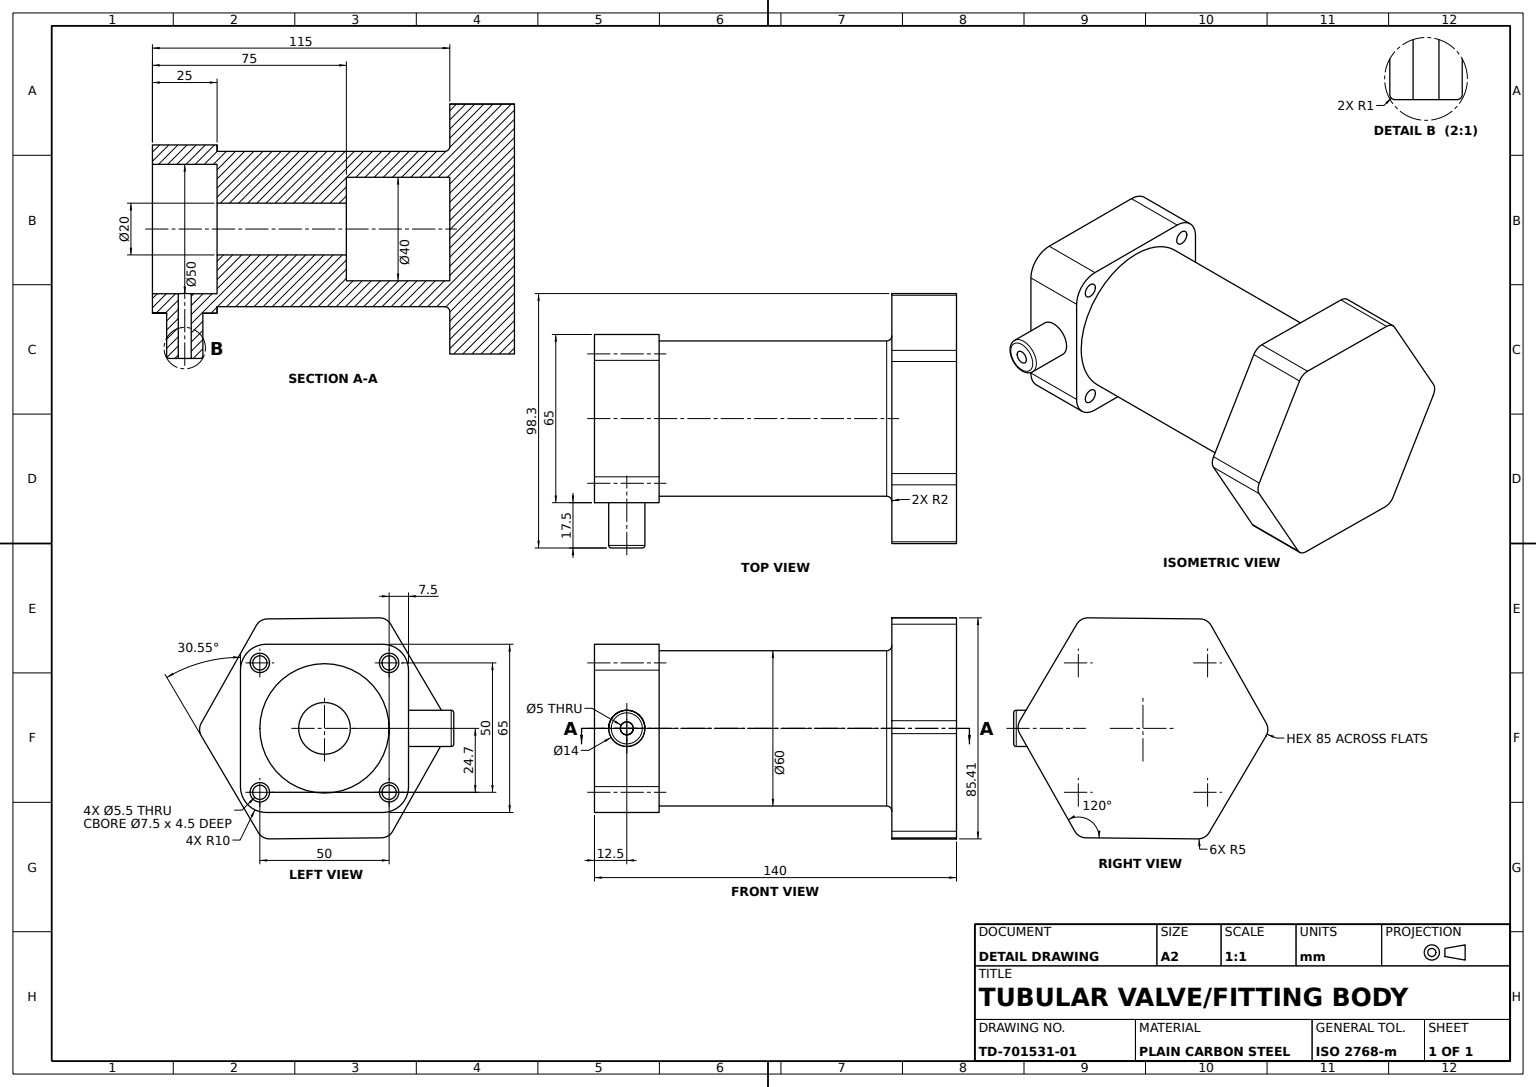
SolidWorks part; units mm, degrees
material "Plain Carbon Steel"
ref_plane "Front Plane" through (0, 0, 0) normal (0, 0, 1) x (1, 0, 0)
ref_plane "Top Plane" through (0, 0, 0) normal (0, 1, 0) x (1, 0, 0)
ref_plane "Right Plane" through (0, 0, 0) normal (1, 0, 0) x (0, 0, -1)
sketch "Hex Profile" plane through (0, 0, 0) normal (0, 0, 1) x (1, 0, 0)
  line L1 (24.1284, 42.7335) -> (-24.9441, 42.2626)
  line L2 (-24.9441, 42.2626) -> (-49.0725, -0.4709)
  line L3 (-49.0725, -0.4709) -> (-24.1284, -42.7335)
  line L4 (-24.1284, -42.7335) -> (24.9441, -42.2626)
  line L5 (24.9441, -42.2626) -> (49.0725, 0.4709)
  line L6 (49.0725, 0.4709) -> (24.1284, 42.7335)
  circle A0 centre (0, 0) radius 42.5 construction
  dimension "D1" = 85
  dimension "D2" = 24.1284
extrude "Hex Body" add sketch "Hex Profile" along normal blind 25
sketch "Body Profile Ø60" plane through (0, 0, 25) normal (0, 0, 1) x (1, 0, 0)
  circle A0 centre (0, 0) radius 30
  dimension "D1" = 60
extrude "Body Cylinder Ø60" add sketch "Body Profile Ø60" along normal blind 90
sketch "Flange Profile 65x65" plane through (0, 0, 115) normal (0, 0, 1) x (1, 0, 0)
  line L1 (-22.5, -32.5) -> (22.5, -32.5)
  line L2 (-32.5, -22.5) -> (-32.5, 22.5)
  line L3 (-22.5, 32.5) -> (22.5, 32.5)
  line L4 (32.5, -22.5) -> (32.5, 22.5)
  line L5 (-32.5, -32.5) -> (32.5, 32.5) construction
  line L6 (-32.5, 32.5) -> (32.5, -32.5) construction
  arc A0 (-22.5, -32.5) -> (-32.5, -22.5) centre (-22.5, -22.5) cw
  arc A1 (22.5, -32.5) -> (32.5, -22.5) centre (22.5, -22.5) ccw
  arc A2 (32.5, 22.5) -> (22.5, 32.5) centre (22.5, 22.5) ccw
  arc A3 (-22.5, 32.5) -> (-32.5, 22.5) centre (-22.5, 22.5) ccw
  point P0 (0, 0)
  dimension "D3" = 10
  dimension "D1" = 65
  dimension "D2" = 65
extrude "Square Flange" add sketch "Flange Profile 65x65" along normal blind 25
sketch "Flange Bore Profile Ø50" plane through (0, 0, 140) normal (0, 0, 1) x (1, 0, 0)
  circle A0 centre (0, 0) radius 25
  dimension "D1" = 50
extrude "Flange Bore Ø50" cut sketch "Flange Bore Profile Ø50" against normal blind 25
sketch "Through Bore Profile Ø20" plane through (0, 0, 115) normal (0, 0, 1) x (1, 0, 0)
  circle A0 centre (0, 0) radius 10
  dimension "D1" = 20
extrude "Through Bore Ø20" cut sketch "Through Bore Profile Ø20" against normal blind 50
sketch "Hex End Bore Profile Ø40" plane through (0, 0, 65) normal (0, 0, 1) x (1, 0, 0)
  circle A0 centre (0, 0) radius 20
  dimension "D1" = 40
extrude "Hex End Bore Ø40" cut sketch "Hex End Bore Profile Ø40" against normal blind 40
fillet "Hex Edge Fillet R5 A" radius 5 1 edges at (24.1284, 42.7335, 12.5)
fillet "Hex Edge Fillet R5 B" radius 5 1 edges at (49.0725, 0.4709, 12.5)
fillet "Hex Edge Fillet R5 C" radius 5 1 edges at (-24.9441, 42.2626, 12.5)
fillet "Hex Edge Fillet R5 D" radius 5 1 edges at (-49.0725, -0.4709, 12.5)
fillet "Hex Edge Fillet R5 E" radius 5 1 edges at (-24.1284, -42.7335, 12.5)
fillet "Hex Edge Fillet R5 F" radius 5 1 edges at (24.9441, -42.2626, 12.5)
sketch "Counterbore Profile 4xØ7.5" plane through (0, 0, 140) normal (0, 0, 1) x (1, 0, 0)
  line L0 (0, 49.1561) -> (0, -58.8104) construction
  circle A1 centre (-25, 25.2951) radius 3.75
  circle A2 centre (-25, -24.7049) radius 3.75
  circle A3 centre (25, -24.7049) radius 3.75
  circle A4 centre (25, 25.2951) radius 3.75
  dimension "D1" = 50
  dimension "D2" = 7.5
  dimension "D3" = 7.5
  dimension "D4" = 50
  dimension "D5" = 50
extrude "Mounting Counterbores 4xØ7.5" cut sketch "Counterbore Profile 4xØ7.5" against normal blind 4.5
sketch "Mounting Hole Profile 4xØ5.5" plane through (0, 0, 135.5) normal (0, 0, 1) x (1, 0, 0)
  circle A0 centre (-25, 25.2951) radius 2.75
  circle A1 centre (25, 25.2951) radius 2.75
  circle A2 centre (25, -24.7049) radius 2.75
  circle A3 centre (-25, -24.7049) radius 2.75
  dimension "D1" = 5.5
  dimension "D2" = 5.5
  dimension "D3" = 5.5
  dimension "D4" = 5.5
extrude "Mounting Holes 4xØ5.5" cut sketch "Mounting Hole Profile 4xØ5.5" against normal blind 20.5
sketch "Port Boss Profile Ø14" plane through (32.5, 0, 0) normal (1, 0, 0) x (0, 0, -1)
  line L0 (-115, -22.5) -> (-115, 22.5) construction
  line L1 (-140, 22.5) -> (-115, 22.5) construction
  circle A1 centre (-127.5, 0) radius 7
  dimension "D1" = 14
  dimension "D2" = 12.5
  dimension "D3" = 22.5
extrude "Pressure Port Boss Ø14" add sketch "Port Boss Profile Ø14" along normal blind 17.5
fillet "Port Boss Tip Fillet R1" radius 1 1 edges at (50, 0, 120.5)
sketch "Port Hole Profile Ø5" plane through (50, 0, 0) normal (1, 0, 0) x (0, 0, -1)
  circle A0 centre (-127.5, 0) radius 2.5
  dimension "D1" = 5
extrude "Port Hole Ø5" cut sketch "Port Hole Profile Ø5" against normal blind 28
fillet "Body to Hex Fillet R2" radius 2 1 edges at (30, 0, 25)
